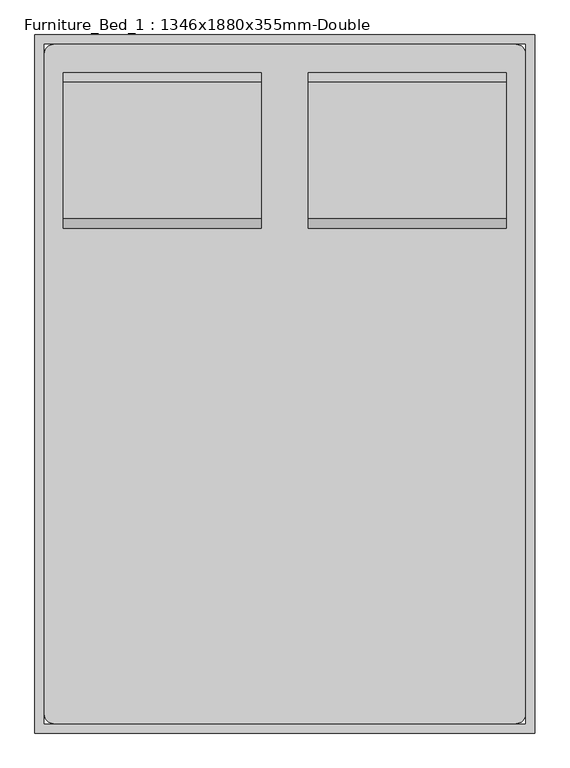
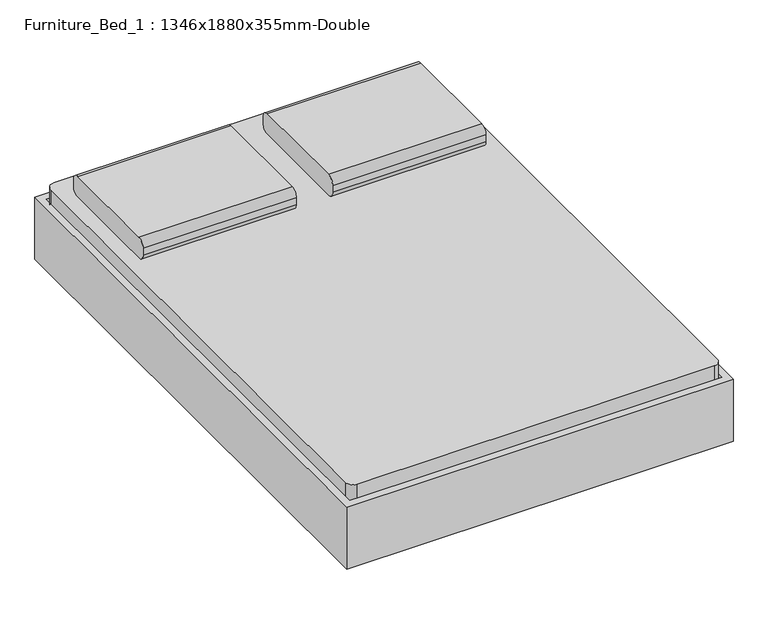
"""IFC4 building model written with IfcOpenShell, lengths in millimetres: furniture geometry, Furniture_Bed_1 : 1346x1880x355mm-Double."""

from ifc_helpers import new_model, si_unit, point, frame, frame_2d, origin, place, context, project, spatial, polyline, circle_curve, trimmed, segment, composite_curve, outline, extrude, source, transform, mapped, element, save
from ifc_brep_helpers import plane_surface, cylinder_surface, revolved_surface, advanced_brep


def furniture_bed_1_1346x1880x355mm_double_93dec6ea(model_context):
    return source(origin(), model_context, "Body", "SolidModel", [
        advanced_brep(
        [(-308.447541, -869.6295082, 196.85), (-308.447541, -869.6295082, 177.8), (-308.447541, -945.8295082, 177.8), (-308.447541, -945.8295082, 196.85), (-245.5113525, -869.6295082, 196.85), (-257.647541, -869.6295082, 177.8), (-257.647541, -945.8295082, 177.8), (-245.5113525, -945.8295082, 196.85), (-164.3115092, -869.6295082, 22.716374), (-181.5766725, -869.6295082, 14.6654962), (-181.5766725, -945.8295082, 14.6654962), (-164.3115092, -945.8295082, 22.716374), (-158.5564547, -869.6295082, 0.0), (-158.5564547, -869.6295082, 19.05), (-158.5564547, -945.8295082, 0.0), (-158.5564547, -945.8295082, 19.05), (-79.9439489, -869.6295082, 19.05), (-79.9439489, -869.6295082, 0.0), (-79.9439489, -945.8295082, 0.0), (-79.9439489, -945.8295082, 19.05), (-67.2439489, -869.6295082, 3.4029547), (-76.7689489, -869.6295082, 19.9007387), (-67.2439489, -945.8295082, 3.4029547), (-76.7689489, -945.8295082, 19.9007387), (-12.2513357, -869.6295082, 57.15), (-7.1469036, -869.6295082, 38.1), (-7.1469036, -945.8295082, 38.1), (-12.2513357, -945.8295082, 57.15), (690.5562537, -869.6295082, 57.15), (685.4518216, -869.6295082, 38.1), (685.4518216, -945.8295082, 38.1), (690.5562537, -945.8295082, 57.15), (755.0738669, -869.6295082, 19.9007387), (745.5488669, -869.6295082, 3.4029547), (745.5488669, -945.8295082, 3.4029547), (755.0738669, -945.8295082, 19.9007387), (758.2488669, -869.6295082, 0.0), (758.2488669, -869.6295082, 19.05), (758.2488669, -945.8295082, 0.0), (758.2488669, -945.8295082, 19.05), (836.8613728, -869.6295082, 19.05), (836.8613728, -869.6295082, 0.0), (836.8613728, -945.8295082, 0.0), (836.8613728, -945.8295082, 19.05), (859.8815906, -869.6295082, 14.6654962), (842.6164272, -869.6295082, 22.716374), (859.8815906, -945.8295082, 14.6654962), (842.6164272, -945.8295082, 22.716374), (923.8162705, -869.6295082, 196.85), (935.952459, -869.6295082, 177.8), (935.952459, -945.8295082, 177.8), (923.8162705, -945.8295082, 196.85), (986.752459, -869.6295082, 196.85), (986.752459, -945.8295082, 196.85), (986.752459, -945.8295082, 177.8), (986.752459, -869.6295082, 177.8)],
        [
            (0, 1),
            (1, 2),
            (2, 3),
            (3, 0),
            (0, 4),
            (4, 5),
            (5, 1),
            (5, 6),
            (6, 2),
            (6, 7),
            (7, 3),
            (7, 4),
            (4, 8),
            (8, 9),
            (9, 5),
            (9, 10),
            (10, 6),
            (10, 11),
            (11, 7),
            (11, 8),
            (12, 9, circle_curve(frame((-158.5564547, -869.6295082, 25.4), z_axis=(0.0, 1.0, 0.0), x_axis=(-0.9063077870366627, 0.0, -0.42261826174067213)), 25.4)),
            (8, 13, circle_curve(frame((-158.5564547, -869.6295082, 25.4), z_axis=(0.0, -1.0, 0.0), x_axis=(-0.9063077870366627, 0.0, -0.42261826174067213)), 6.35)),
            (13, 12),
            (14, 10, circle_curve(frame((-158.5564547, -945.8295082, 25.4), z_axis=(0.0, 1.0, 0.0), x_axis=(-0.9063077870366627, 0.0, -0.42261826174067213)), 25.4)),
            (12, 14),
            (15, 11, circle_curve(frame((-158.5564547, -945.8295082, 25.4), z_axis=(0.0, 1.0, 0.0), x_axis=(-0.9063077870366627, 0.0, -0.42261826174067213)), 6.35)),
            (14, 15),
            (15, 13),
            (13, 16),
            (16, 17),
            (17, 12),
            (17, 18),
            (18, 14),
            (18, 19),
            (19, 15),
            (19, 16),
            (20, 17, circle_curve(frame((-79.9439489, -869.6295082, 25.4), z_axis=(0.0, 1.0, 0.0), x_axis=(0.0, 0.0, -1.0)), 25.4)),
            (16, 21, circle_curve(frame((-79.9439489, -869.6295082, 25.4), z_axis=(0.0, -1.0, 0.0), x_axis=(0.0, 0.0, -1.0)), 6.35)),
            (21, 20),
            (22, 18, circle_curve(frame((-79.9439489, -945.8295082, 25.4), z_axis=(0.0, 1.0, 0.0), x_axis=(0.0, 0.0, -1.0)), 25.4)),
            (20, 22),
            (23, 19, circle_curve(frame((-79.9439489, -945.8295082, 25.4), z_axis=(0.0, 1.0, 0.0), x_axis=(0.0, 0.0, -1.0)), 6.35)),
            (22, 23),
            (23, 21),
            (21, 24),
            (24, 25),
            (25, 20),
            (25, 26),
            (26, 22),
            (26, 27),
            (27, 23),
            (27, 24),
            (24, 28),
            (28, 29),
            (29, 25),
            (29, 30),
            (30, 26),
            (30, 31),
            (31, 27),
            (31, 28),
            (28, 32),
            (32, 33),
            (33, 29),
            (33, 34),
            (34, 30),
            (34, 35),
            (35, 31),
            (35, 32),
            (36, 33, circle_curve(frame((758.2488669, -869.6295082, 25.4), z_axis=(0.0, 1.0, 0.0), x_axis=(-0.5000000000000486, 0.0, -0.8660254037844105)), 25.4)),
            (32, 37, circle_curve(frame((758.2488669, -869.6295082, 25.4), z_axis=(0.0, -1.0, 0.0), x_axis=(-0.5000000000000486, 0.0, -0.8660254037844105)), 6.35)),
            (37, 36),
            (38, 34, circle_curve(frame((758.2488669, -945.8295082, 25.4), z_axis=(0.0, 1.0, 0.0), x_axis=(-0.5000000000000486, 0.0, -0.8660254037844105)), 25.4)),
            (36, 38),
            (39, 35, circle_curve(frame((758.2488669, -945.8295082, 25.4), z_axis=(0.0, 1.0, 0.0), x_axis=(-0.5000000000000486, 0.0, -0.8660254037844105)), 6.35)),
            (38, 39),
            (39, 37),
            (37, 40),
            (40, 41),
            (41, 36),
            (41, 42),
            (42, 38),
            (42, 43),
            (43, 39),
            (43, 40),
            (44, 41, circle_curve(frame((836.8613728, -869.6295082, 25.4), z_axis=(0.0, 1.0, 0.0), x_axis=(0.0, 0.0, -1.0)), 25.4)),
            (40, 45, circle_curve(frame((836.8613728, -869.6295082, 25.4), z_axis=(0.0, -1.0, 0.0), x_axis=(0.0, 0.0, -1.0)), 6.35)),
            (45, 44),
            (46, 42, circle_curve(frame((836.8613728, -945.8295082, 25.4), z_axis=(0.0, 1.0, 0.0), x_axis=(0.0, 0.0, -1.0)), 25.4)),
            (44, 46),
            (47, 43, circle_curve(frame((836.8613728, -945.8295082, 25.4), z_axis=(0.0, 1.0, 0.0), x_axis=(0.0, 0.0, -1.0)), 6.35)),
            (46, 47),
            (47, 45),
            (45, 48),
            (48, 49),
            (49, 44),
            (49, 50),
            (50, 46),
            (50, 51),
            (51, 47),
            (51, 48),
            (52, 53),
            (53, 54),
            (54, 55),
            (55, 52),
            (48, 52),
            (55, 49),
            (54, 50),
            (53, 51),
        ],
        [
            plane_surface(frame((-308.447541, -1174.4295082, -127.5947323), z_axis=(-1.0, 0.0, 0.0), x_axis=(0.0, 1.0, 0.0))),
            plane_surface(frame((-308.447541, -869.6295082, 196.85), z_axis=(0.0, 1.0, 0.0), x_axis=(1.0, 0.0, 0.0))),
            plane_surface(frame((-308.447541, -869.6295082, 177.8), z_axis=(0.0, 0.0, -1.0), x_axis=(1.0, 0.0, 0.0))),
            plane_surface(frame((-308.447541, -945.8295082, 177.8), z_axis=(0.0, -1.0, 0.0), x_axis=(1.0, 0.0, 0.0))),
            plane_surface(frame((-308.447541, -945.8295082, 196.85), z_axis=(0.0, 0.0, 1.0), x_axis=(1.0, 0.0, 0.0))),
            plane_surface(frame((-245.5113525, -869.6295082, 196.85), z_axis=(0.0, 1.0, 0.0), x_axis=(0.42261826174067146, 0.0, -0.906307787036663))),
            plane_surface(frame((-257.647541, -869.6295082, 177.8), z_axis=(-0.9063077870366631, 0.0, -0.4226182617406713), x_axis=(0.4226182617406713, 0.0, -0.9063077870366631))),
            plane_surface(frame((-257.647541, -945.8295082, 177.8), z_axis=(0.0, -1.0, 0.0), x_axis=(0.4226182617406716, 0.0, -0.9063077870366629))),
            plane_surface(frame((-245.5113525, -945.8295082, 196.85), z_axis=(0.906307787036663, 0.0, 0.4226182617406716), x_axis=(0.4226182617406716, 0.0, -0.906307787036663))),
            plane_surface(frame((-158.5564547, -869.6295082, 25.4), z_axis=(0.0, 1.0, 0.0), x_axis=(-0.9063077870366627, 0.0, -0.42261826174067213))),
            cylinder_surface(frame((-158.5564547, -1174.4295082, 25.4), z_axis=(0.0, -1.0, 0.0), x_axis=(-0.9063077870366627, 0.0, -0.42261826174067213)), 25.4),
            plane_surface(frame((-158.5564547, -945.8295082, 25.4), z_axis=(0.0, -1.0, 0.0), x_axis=(-0.9063077870366627, 0.0, -0.42261826174067213))),
            revolved_surface(polyline([(-164.31150914768278, -945.8295082, 22.716374037946732), (-164.31150914768278, -869.6295082, 22.716374037946732)]), (-158.5564547, -1174.4295082, 25.4), (0.0, -1.0, 0.0)),
            plane_surface(frame((-158.5564547, -869.6295082, 19.05), z_axis=(0.0, 1.0, 0.0), x_axis=(1.0, 0.0, 0.0))),
            plane_surface(frame((-158.5564547, -869.6295082, 0.0), z_axis=(0.0, 0.0, -1.0), x_axis=(1.0, 0.0, 0.0))),
            plane_surface(frame((-158.5564547, -945.8295082, 0.0), z_axis=(0.0, -1.0, 0.0), x_axis=(1.0, 0.0, 0.0))),
            plane_surface(frame((-158.5564547, -945.8295082, 19.05), z_axis=(0.0, 0.0, 1.0), x_axis=(1.0, 0.0, 0.0))),
            plane_surface(frame((-79.9439489, -869.6295082, 25.4), z_axis=(0.0, 1.0, 0.0), x_axis=(0.0, 0.0, -1.0))),
            cylinder_surface(frame((-79.9439489, -1174.4295082, 25.4), z_axis=(0.0, -1.0, 0.0), x_axis=(0.0, 0.0, -1.0)), 25.4),
            plane_surface(frame((-79.9439489, -945.8295082, 25.4), z_axis=(0.0, -1.0, 0.0), x_axis=(0.0, 0.0, -1.0))),
            revolved_surface(polyline([(-79.9439489, -945.8295082, 19.049999999999997), (-79.9439489, -869.6295082, 19.049999999999997)]), (-79.9439489, -1174.4295082, 25.4), (0.0, -1.0, 0.0)),
            plane_surface(frame((-76.7689489, -869.6295082, 19.9007387), z_axis=(0.0, 1.0, 0.0), x_axis=(0.8660254037844782, 0.0, 0.4999999999999314))),
            plane_surface(frame((-67.2439489, -869.6295082, 3.4029547), z_axis=(0.49999999999993133, 0.0, -0.8660254037844783), x_axis=(0.8660254037844783, 0.0, 0.49999999999993133))),
            plane_surface(frame((-67.2439489, -945.8295082, 3.4029547), z_axis=(0.0, -1.0, 0.0), x_axis=(0.8660254037844785, 0.0, 0.499999999999931))),
            plane_surface(frame((-76.7689489, -945.8295082, 19.9007387), z_axis=(-0.49999999999993144, 0.0, 0.8660254037844782), x_axis=(0.8660254037844782, 0.0, 0.49999999999993144))),
            plane_surface(frame((-12.2513357, -869.6295082, 57.15), z_axis=(0.0, 1.0, 0.0), x_axis=(1.0, 0.0, 0.0))),
            plane_surface(frame((-7.1469036, -869.6295082, 38.1), z_axis=(0.0, 0.0, -1.0), x_axis=(1.0, 0.0, 0.0))),
            plane_surface(frame((-7.1469036, -945.8295082, 38.1), z_axis=(0.0, -1.0, 0.0), x_axis=(1.0, 0.0, 0.0))),
            plane_surface(frame((-12.2513357, -945.8295082, 57.15), z_axis=(0.0, 0.0, 1.0), x_axis=(1.0, 0.0, 0.0))),
            plane_surface(frame((690.5562537, -869.6295082, 57.15), z_axis=(0.0, 1.0, 0.0), x_axis=(0.8660254037844104, 0.0, -0.5000000000000491))),
            plane_surface(frame((685.4518216, -869.6295082, 38.1), z_axis=(-0.5000000000000484, 0.0, -0.8660254037844108), x_axis=(0.8660254037844108, 0.0, -0.5000000000000484))),
            plane_surface(frame((685.4518216, -945.8295082, 38.1), z_axis=(0.0, -1.0000000000000002, 0.0), x_axis=(0.8660254037844103, 0.0, -0.5000000000000493))),
            plane_surface(frame((690.5562537, -945.8295082, 57.15), z_axis=(0.5000000000000485, 0.0, 0.8660254037844106), x_axis=(0.8660254037844106, 0.0, -0.5000000000000485))),
            plane_surface(frame((758.2488669, -869.6295082, 25.4), z_axis=(0.0, 1.0000000000000002, 0.0), x_axis=(-0.5000000000000487, 0.0, -0.8660254037844106))),
            cylinder_surface(frame((758.2488669, -1174.4295082, 25.4), z_axis=(0.0, -1.0, 0.0), x_axis=(-0.5000000000000486, 0.0, -0.8660254037844105)), 25.4),
            plane_surface(frame((758.2488669, -945.8295082, 25.4), z_axis=(0.0, -1.0000000000000002, 0.0), x_axis=(-0.5000000000000487, 0.0, -0.8660254037844106))),
            revolved_surface(polyline([(755.0738668999998, -945.8295082, 19.900738685968992), (755.0738668999998, -869.6295082, 19.900738685968992)]), (758.2488669, -1174.4295082, 25.4), (0.0, -1.0, 0.0)),
            plane_surface(frame((758.2488669, -869.6295082, 19.05), z_axis=(0.0, 1.0, 0.0), x_axis=(1.0, 0.0, 0.0))),
            plane_surface(frame((758.2488669, -869.6295082, 0.0), z_axis=(0.0, 0.0, -1.0), x_axis=(1.0, 0.0, 0.0))),
            plane_surface(frame((758.2488669, -945.8295082, 0.0), z_axis=(0.0, -1.0, 0.0), x_axis=(1.0, 0.0, 0.0))),
            plane_surface(frame((758.2488669, -945.8295082, 19.05), z_axis=(0.0, 0.0, 1.0), x_axis=(1.0, 0.0, 0.0))),
            plane_surface(frame((836.8613728, -869.6295082, 25.4), z_axis=(0.0, 1.0, 0.0), x_axis=(0.0, 0.0, -1.0))),
            cylinder_surface(frame((836.8613728, -1174.4295082, 25.4), z_axis=(0.0, -1.0, 0.0), x_axis=(0.0, 0.0, -1.0)), 25.4),
            plane_surface(frame((836.8613728, -945.8295082, 25.4), z_axis=(0.0, -1.0, 0.0), x_axis=(0.0, 0.0, -1.0))),
            revolved_surface(polyline([(836.8613728, -945.8295082, 19.049999999999997), (836.8613728, -869.6295082, 19.049999999999997)]), (836.8613728, -1174.4295082, 25.4), (0.0, -1.0, 0.0)),
            plane_surface(frame((842.6164272, -869.6295082, 22.716374), z_axis=(0.0, 1.0, 0.0), x_axis=(0.4226182617405402, 0.0, 0.9063077870367242))),
            plane_surface(frame((859.8815906, -869.6295082, 14.6654962), z_axis=(0.9063077870367245, 0.0, -0.42261826174053974), x_axis=(0.42261826174053974, 0.0, 0.9063077870367245))),
            plane_surface(frame((859.8815906, -945.8295082, 14.6654962), z_axis=(0.0, -1.0000000000000002, 0.0), x_axis=(0.42261826174053974, 0.0, 0.9063077870367245))),
            plane_surface(frame((842.6164272, -945.8295082, 22.716374), z_axis=(-0.9063077870367247, 0.0, 0.4226182617405394), x_axis=(0.4226182617405394, 0.0, 0.9063077870367247))),
            plane_surface(frame((986.752459, -1174.4295082, -127.5947323), z_axis=(1.0, 0.0, 0.0), x_axis=(0.0, 1.0, 0.0))),
            plane_surface(frame((923.8162705, -869.6295082, 196.85), z_axis=(0.0, 1.0, 0.0), x_axis=(1.0, 0.0, 0.0))),
            plane_surface(frame((935.952459, -869.6295082, 177.8), z_axis=(0.0, 0.0, -1.0), x_axis=(1.0, 0.0, 0.0))),
            plane_surface(frame((935.952459, -945.8295082, 177.8), z_axis=(0.0, -1.0, 0.0), x_axis=(1.0, 0.0, 0.0))),
            plane_surface(frame((923.8162705, -945.8295082, 196.85), z_axis=(0.0, 0.0, 1.0), x_axis=(1.0, 0.0, 0.0))),
        ],
        [
            (0, [[1, 2, 3, 4]]),
            (1, [[-1, 5, 6, 7]]),
            (2, [[-2, -7, 8, 9]]),
            (3, [[-3, -9, 10, 11]]),
            (4, [[-4, -11, 12, -5]]),
            (5, [[-6, 13, 14, 15]]),
            (6, [[-8, -15, 16, 17]]),
            (7, [[-10, -17, 18, 19]]),
            (8, [[-12, -19, 20, -13]]),
            (9, [[21, -14, 22, 23]]),
            (10, [[24, -16, -21, 25]]),
            (11, [[26, -18, -24, 27]]),
            (12, [[-22, -20, -26, 28]]),
            (13, [[-23, 29, 30, 31]]),
            (14, [[-25, -31, 32, 33]]),
            (15, [[-27, -33, 34, 35]]),
            (16, [[-28, -35, 36, -29]]),
            (17, [[37, -30, 38, 39]]),
            (18, [[40, -32, -37, 41]]),
            (19, [[42, -34, -40, 43]]),
            (20, [[-38, -36, -42, 44]]),
            (21, [[-39, 45, 46, 47]]),
            (22, [[-41, -47, 48, 49]]),
            (23, [[-43, -49, 50, 51]]),
            (24, [[-44, -51, 52, -45]]),
            (25, [[-46, 53, 54, 55]]),
            (26, [[-48, -55, 56, 57]]),
            (27, [[-50, -57, 58, 59]]),
            (28, [[-52, -59, 60, -53]]),
            (29, [[-54, 61, 62, 63]]),
            (30, [[-56, -63, 64, 65]]),
            (31, [[-58, -65, 66, 67]]),
            (32, [[-60, -67, 68, -61]]),
            (33, [[69, -62, 70, 71]]),
            (34, [[72, -64, -69, 73]]),
            (35, [[74, -66, -72, 75]]),
            (36, [[-70, -68, -74, 76]]),
            (37, [[-71, 77, 78, 79]]),
            (38, [[-73, -79, 80, 81]]),
            (39, [[-75, -81, 82, 83]]),
            (40, [[-76, -83, 84, -77]]),
            (41, [[85, -78, 86, 87]]),
            (42, [[88, -80, -85, 89]]),
            (43, [[90, -82, -88, 91]]),
            (44, [[-86, -84, -90, 92]]),
            (45, [[-87, 93, 94, 95]]),
            (46, [[-89, -95, 96, 97]]),
            (47, [[-91, -97, 98, 99]]),
            (48, [[-92, -99, 100, -93]]),
            (49, [[101, 102, 103, 104]]),
            (50, [[-94, 105, -104, 106]]),
            (51, [[-96, -106, -103, 107]]),
            (52, [[-98, -107, -102, 108]]),
            (53, [[-100, -108, -101, -105]]),
        ],
    ),
        extrude(outline(composite_curve([segment(polyline([(-283.047541, 680.1704918), (961.352459, 680.1704918)]), True, "CONTINUOUS"), segment(trimmed(circle_curve(frame_2d((961.352459, 654.7704918)), 25.4), [point((961.352459, 680.1704918))], [point((986.752459, 654.7704918))], False, "CARTESIAN"), True, "CONTINUOUS"), segment(polyline([(986.752459, 654.7704918), (986.752459, -1123.6295082)]), True, "CONTINUOUS"), segment(trimmed(circle_curve(frame_2d((961.352459, -1123.6295082)), 25.4), [point((986.752459, -1123.6295082))], [point((961.352459, -1149.0295082))], False, "CARTESIAN"), True, "CONTINUOUS"), segment(polyline([(961.352459, -1149.0295082), (-283.047541, -1149.0295082)]), True, "CONTINUOUS"), segment(trimmed(circle_curve(frame_2d((-283.047541, -1123.6295082)), 25.4), [point((-283.047541, -1149.0295082))], [point((-308.447541, -1123.6295082))], False, "CARTESIAN"), True, "CONTINUOUS"), segment(polyline([(-308.447541, -1123.6295082), (-308.447541, 654.7704918)]), True, "CONTINUOUS"), segment(trimmed(circle_curve(frame_2d((-283.047541, 654.7704918)), 25.4), [point((-308.447541, 654.7704918))], [point((-283.047541, 680.1704918))], False, "CARTESIAN"), True, "CONTINUOUS")], self_intersect=False)), frame((0.0, 0.0, 203.2), z_axis=(0.0, 0.0, 1.0), x_axis=(1.0, 0.0, 0.0)), (0.0, 0.0, 1.0), 203.2),
        advanced_brep(
        [(-308.1231784, 451.5704918, 177.8), (-308.1231784, 375.3704918, 177.8), (-308.1231784, 375.3704918, 196.85), (-308.1231784, 451.5704918, 196.85), (-257.3231784, 451.5704918, 177.8), (-257.3231784, 375.3704918, 177.8), (-245.1869899, 375.3704918, 196.85), (-245.1869899, 451.5704918, 196.85), (-181.2523099, 451.5704918, 14.6654962), (-181.2523099, 375.3704918, 14.6654962), (-163.9871466, 375.3704918, 22.716374), (-163.9871466, 451.5704918, 22.716374), (-158.2320921, 375.3704918, 0.0), (-158.2320921, 451.5704918, 0.0), (-158.2320921, 375.3704918, 19.05), (-158.2320921, 451.5704918, 19.05), (-79.6195862, 451.5704918, 0.0), (-79.6195862, 375.3704918, 0.0), (-79.6195862, 375.3704918, 19.05), (-79.6195862, 451.5704918, 19.05), (-66.9195862, 375.3704918, 3.4029547), (-66.9195862, 451.5704918, 3.4029547), (-76.4445862, 375.3704918, 19.9007387), (-76.4445862, 451.5704918, 19.9007387), (-6.822541, 451.5704918, 38.1), (-6.822541, 375.3704918, 38.1), (-11.9269731, 375.3704918, 57.15), (-11.9269731, 451.5704918, 57.15), (685.4518216, 451.5704918, 38.1), (685.4518216, 375.3704918, 38.1), (690.5562537, 375.3704918, 57.15), (690.5562537, 451.5704918, 57.15), (745.5488669, 451.5704918, 3.4029547), (745.5488669, 375.3704918, 3.4029547), (755.0738669, 375.3704918, 19.9007387), (755.0738669, 451.5704918, 19.9007387), (758.2488669, 375.3704918, 0.0), (758.2488669, 451.5704918, 0.0), (758.2488669, 375.3704918, 19.05), (758.2488669, 451.5704918, 19.05), (836.8613728, 451.5704918, 0.0), (836.8613728, 375.3704918, 0.0), (836.8613728, 375.3704918, 19.05), (836.8613728, 451.5704918, 19.05), (859.8815906, 375.3704918, 14.6654962), (859.8815906, 451.5704918, 14.6654962), (842.6164272, 375.3704918, 22.716374), (842.6164272, 451.5704918, 22.716374), (935.952459, 451.5704918, 177.8), (935.952459, 375.3704918, 177.8), (923.8162705, 375.3704918, 196.85), (923.8162705, 451.5704918, 196.85), (986.752459, 451.5704918, 177.8), (986.752459, 451.5704918, 196.85), (986.752459, 375.3704918, 196.85), (986.752459, 375.3704918, 177.8)],
        [
            (0, 1),
            (1, 2),
            (2, 3),
            (3, 0),
            (0, 4),
            (4, 5),
            (5, 1),
            (5, 6),
            (6, 2),
            (6, 7),
            (7, 3),
            (7, 4),
            (4, 8),
            (8, 9),
            (9, 5),
            (9, 10),
            (10, 6),
            (10, 11),
            (11, 7),
            (11, 8),
            (12, 9, circle_curve(frame((-158.2320921, 375.3704918, 25.4), z_axis=(0.0, 1.0, 0.0), x_axis=(-0.906307787036649, 0.0, -0.4226182617407015)), 25.4)),
            (8, 13, circle_curve(frame((-158.2320921, 451.5704918, 25.4), z_axis=(0.0, -1.0, 0.0), x_axis=(-0.906307787036649, 0.0, -0.4226182617407015)), 25.4)),
            (13, 12),
            (14, 10, circle_curve(frame((-158.2320921, 375.3704918, 25.4), z_axis=(0.0, 1.0, 0.0), x_axis=(-0.906307787036649, 0.0, -0.4226182617407015)), 6.35)),
            (12, 14),
            (15, 11, circle_curve(frame((-158.2320921, 451.5704918, 25.4), z_axis=(0.0, 1.0, 0.0), x_axis=(-0.906307787036649, 0.0, -0.4226182617407015)), 6.35)),
            (14, 15),
            (15, 13),
            (13, 16),
            (16, 17),
            (17, 12),
            (17, 18),
            (18, 14),
            (18, 19),
            (19, 15),
            (19, 16),
            (20, 17, circle_curve(frame((-79.6195862, 375.3704918, 25.4), z_axis=(0.0, 1.0, 0.0), x_axis=(0.0, 0.0, -1.0)), 25.4)),
            (16, 21, circle_curve(frame((-79.6195862, 451.5704918, 25.4), z_axis=(0.0, -1.0, 0.0), x_axis=(0.0, 0.0, -1.0)), 25.4)),
            (21, 20),
            (22, 18, circle_curve(frame((-79.6195862, 375.3704918, 25.4), z_axis=(0.0, 1.0, 0.0), x_axis=(0.0, 0.0, -1.0)), 6.35)),
            (20, 22),
            (23, 19, circle_curve(frame((-79.6195862, 451.5704918, 25.4), z_axis=(0.0, 1.0, 0.0), x_axis=(0.0, 0.0, -1.0)), 6.35)),
            (22, 23),
            (23, 21),
            (21, 24),
            (24, 25),
            (25, 20),
            (25, 26),
            (26, 22),
            (26, 27),
            (27, 23),
            (27, 24),
            (24, 28),
            (28, 29),
            (29, 25),
            (29, 30),
            (30, 26),
            (30, 31),
            (31, 27),
            (31, 28),
            (28, 32),
            (32, 33),
            (33, 29),
            (33, 34),
            (34, 30),
            (34, 35),
            (35, 31),
            (35, 32),
            (36, 33, circle_curve(frame((758.2488669, 375.3704918, 25.4), z_axis=(0.0, 1.0, 0.0), x_axis=(-0.5000000000000444, 0.0, -0.866025403784413)), 25.4)),
            (32, 37, circle_curve(frame((758.2488669, 451.5704918, 25.4), z_axis=(0.0, -1.0, 0.0), x_axis=(-0.5000000000000444, 0.0, -0.866025403784413)), 25.4)),
            (37, 36),
            (38, 34, circle_curve(frame((758.2488669, 375.3704918, 25.4), z_axis=(0.0, 1.0, 0.0), x_axis=(-0.5000000000000444, 0.0, -0.866025403784413)), 6.35)),
            (36, 38),
            (39, 35, circle_curve(frame((758.2488669, 451.5704918, 25.4), z_axis=(0.0, 1.0, 0.0), x_axis=(-0.5000000000000444, 0.0, -0.866025403784413)), 6.35)),
            (38, 39),
            (39, 37),
            (37, 40),
            (40, 41),
            (41, 36),
            (41, 42),
            (42, 38),
            (42, 43),
            (43, 39),
            (43, 40),
            (44, 41, circle_curve(frame((836.8613728, 375.3704918, 25.4), z_axis=(0.0, 1.0, 0.0), x_axis=(0.0, 0.0, -1.0)), 25.4)),
            (40, 45, circle_curve(frame((836.8613728, 451.5704918, 25.4), z_axis=(0.0, -1.0, 0.0), x_axis=(0.0, 0.0, -1.0)), 25.4)),
            (45, 44),
            (46, 42, circle_curve(frame((836.8613728, 375.3704918, 25.4), z_axis=(0.0, 1.0, 0.0), x_axis=(0.0, 0.0, -1.0)), 6.35)),
            (44, 46),
            (47, 43, circle_curve(frame((836.8613728, 451.5704918, 25.4), z_axis=(0.0, 1.0, 0.0), x_axis=(0.0, 0.0, -1.0)), 6.35)),
            (46, 47),
            (47, 45),
            (45, 48),
            (48, 49),
            (49, 44),
            (49, 50),
            (50, 46),
            (50, 51),
            (51, 47),
            (51, 48),
            (52, 53),
            (53, 54),
            (54, 55),
            (55, 52),
            (48, 52),
            (55, 49),
            (54, 50),
            (53, 51),
        ],
        [
            plane_surface(frame((-308.1231784, 705.5704918, -152.9490627), z_axis=(-1.0, 0.0, 0.0), x_axis=(0.0, 1.0, 0.0))),
            plane_surface(frame((-308.1231784, 451.5704918, 177.8), z_axis=(0.0, 0.0, -1.0), x_axis=(1.0, 0.0, 0.0))),
            plane_surface(frame((-308.1231784, 375.3704918, 177.8), z_axis=(0.0, -1.0, 0.0), x_axis=(1.0, 0.0, 0.0))),
            plane_surface(frame((-308.1231784, 375.3704918, 196.85), z_axis=(0.0, 0.0, 1.0), x_axis=(1.0, 0.0, 0.0))),
            plane_surface(frame((-308.1231784, 451.5704918, 196.85), z_axis=(0.0, 1.0, 0.0), x_axis=(1.0, 0.0, 0.0))),
            plane_surface(frame((-257.3231784, 451.5704918, 177.8), z_axis=(-0.9063077870366483, 0.0, -0.4226182617407031), x_axis=(0.4226182617407031, 0.0, -0.9063077870366483))),
            plane_surface(frame((-257.3231784, 375.3704918, 177.8), z_axis=(0.0, -1.0, 0.0), x_axis=(0.4226182617407027, 0.0, -0.9063077870366485))),
            plane_surface(frame((-245.1869899, 375.3704918, 196.85), z_axis=(0.9063077870366484, 0.0, 0.4226182617407029), x_axis=(0.4226182617407029, 0.0, -0.9063077870366484))),
            plane_surface(frame((-245.1869899, 451.5704918, 196.85), z_axis=(0.0, 1.0, 0.0), x_axis=(0.4226182617407027, 0.0, -0.9063077870366485))),
            cylinder_surface(frame((-158.2320921, 705.5704918, 25.4), z_axis=(0.0, -1.0, 0.0), x_axis=(-0.906307787036649, 0.0, -0.4226182617407015)), 25.4),
            plane_surface(frame((-158.2320921, 375.3704918, 25.4), z_axis=(0.0, -1.0, 0.0), x_axis=(-0.906307787036649, 0.0, -0.4226182617407015))),
            revolved_surface(polyline([(-163.9871465476827, 375.3704918, 22.716374037946544), (-163.9871465476827, 451.5704918, 22.716374037946544)]), (-158.2320921, 705.5704918, 25.4), (0.0, -1.0, 0.0)),
            plane_surface(frame((-158.2320921, 451.5704918, 25.4), z_axis=(0.0, 1.0, 0.0), x_axis=(-0.906307787036649, 0.0, -0.4226182617407015))),
            plane_surface(frame((-158.2320921, 451.5704918, 0.0), z_axis=(0.0, 0.0, -1.0), x_axis=(1.0, 0.0, 0.0))),
            plane_surface(frame((-158.2320921, 375.3704918, 0.0), z_axis=(0.0, -1.0, 0.0), x_axis=(1.0, 0.0, 0.0))),
            plane_surface(frame((-158.2320921, 375.3704918, 19.05), z_axis=(0.0, 0.0, 1.0), x_axis=(1.0, 0.0, 0.0))),
            plane_surface(frame((-158.2320921, 451.5704918, 19.05), z_axis=(0.0, 1.0, 0.0), x_axis=(1.0, 0.0, 0.0))),
            cylinder_surface(frame((-79.6195862, 705.5704918, 25.4), z_axis=(0.0, -1.0, 0.0), x_axis=(0.0, 0.0, -1.0)), 25.4),
            plane_surface(frame((-79.6195862, 375.3704918, 25.4), z_axis=(0.0, -1.0, 0.0), x_axis=(0.0, 0.0, -1.0))),
            revolved_surface(polyline([(-79.6195862, 375.3704918, 19.049999999999997), (-79.6195862, 451.5704918, 19.049999999999997)]), (-79.6195862, 705.5704918, 25.4), (0.0, -1.0, 0.0)),
            plane_surface(frame((-79.6195862, 451.5704918, 25.4), z_axis=(0.0, 1.0, 0.0), x_axis=(0.0, 0.0, -1.0))),
            plane_surface(frame((-66.9195862, 451.5704918, 3.4029547), z_axis=(0.4999999999998771, 0.0, -0.8660254037845097), x_axis=(0.8660254037845097, 0.0, 0.4999999999998771))),
            plane_surface(frame((-66.9195862, 375.3704918, 3.4029547), z_axis=(0.0, -1.0000000000000002, 0.0), x_axis=(0.8660254037845102, 0.0, 0.49999999999987627))),
            plane_surface(frame((-76.4445862, 375.3704918, 19.9007387), z_axis=(-0.49999999999987643, 0.0, 0.86602540378451), x_axis=(0.86602540378451, 0.0, 0.49999999999987643))),
            plane_surface(frame((-76.4445862, 451.5704918, 19.9007387), z_axis=(0.0, 1.0, 0.0), x_axis=(0.8660254037845102, 0.0, 0.4999999999998761))),
            plane_surface(frame((-6.822541, 451.5704918, 38.1), z_axis=(0.0, 0.0, -1.0), x_axis=(1.0, 0.0, 0.0))),
            plane_surface(frame((-6.822541, 375.3704918, 38.1), z_axis=(0.0, -1.0, 0.0), x_axis=(1.0, 0.0, 0.0))),
            plane_surface(frame((-11.9269731, 375.3704918, 57.15), z_axis=(0.0, 0.0, 1.0), x_axis=(1.0, 0.0, 0.0))),
            plane_surface(frame((-11.9269731, 451.5704918, 57.15), z_axis=(0.0, 1.0, 0.0), x_axis=(1.0, 0.0, 0.0))),
            plane_surface(frame((685.4518216, 451.5704918, 38.1), z_axis=(-0.5000000000000445, 0.0, -0.866025403784413), x_axis=(0.866025403784413, 0.0, -0.5000000000000445))),
            plane_surface(frame((685.4518216, 375.3704918, 38.1), z_axis=(0.0, -1.0, 0.0), x_axis=(0.8660254037844118, 0.0, -0.5000000000000464))),
            plane_surface(frame((690.5562537, 375.3704918, 57.15), z_axis=(0.5000000000000461, 0.0, 0.8660254037844121), x_axis=(0.8660254037844121, 0.0, -0.5000000000000461))),
            plane_surface(frame((690.5562537, 451.5704918, 57.15), z_axis=(0.0, 1.0, 0.0), x_axis=(0.8660254037844126, 0.0, -0.5000000000000452))),
            cylinder_surface(frame((758.2488669, 705.5704918, 25.4), z_axis=(0.0, -1.0, 0.0), x_axis=(-0.5000000000000444, 0.0, -0.866025403784413)), 25.4),
            plane_surface(frame((758.2488669, 375.3704918, 25.4), z_axis=(0.0, -1.0000000000000002, 0.0), x_axis=(-0.5000000000000445, 0.0, -0.8660254037844131))),
            revolved_surface(polyline([(755.0738668999998, 375.3704918, 19.900738685968975), (755.0738668999998, 451.5704918, 19.900738685968975)]), (758.2488669, 705.5704918, 25.4), (0.0, -1.0, 0.0)),
            plane_surface(frame((758.2488669, 451.5704918, 25.4), z_axis=(0.0, 1.0000000000000002, 0.0), x_axis=(-0.5000000000000445, 0.0, -0.8660254037844131))),
            plane_surface(frame((758.2488669, 451.5704918, 0.0), z_axis=(0.0, 0.0, -1.0), x_axis=(1.0, 0.0, 0.0))),
            plane_surface(frame((758.2488669, 375.3704918, 0.0), z_axis=(0.0, -1.0, 0.0), x_axis=(1.0, 0.0, 0.0))),
            plane_surface(frame((758.2488669, 375.3704918, 19.05), z_axis=(0.0, 0.0, 1.0), x_axis=(1.0, 0.0, 0.0))),
            plane_surface(frame((758.2488669, 451.5704918, 19.05), z_axis=(0.0, 1.0, 0.0), x_axis=(1.0, 0.0, 0.0))),
            cylinder_surface(frame((836.8613728, 705.5704918, 25.4), z_axis=(0.0, -1.0, 0.0), x_axis=(0.0, 0.0, -1.0)), 25.4),
            plane_surface(frame((836.8613728, 375.3704918, 25.4), z_axis=(0.0, -1.0, 0.0), x_axis=(0.0, 0.0, -1.0))),
            revolved_surface(polyline([(836.8613728, 375.3704918, 19.049999999999997), (836.8613728, 451.5704918, 19.049999999999997)]), (836.8613728, 705.5704918, 25.4), (0.0, -1.0, 0.0)),
            plane_surface(frame((836.8613728, 451.5704918, 25.4), z_axis=(0.0, 1.0, 0.0), x_axis=(0.0, 0.0, -1.0))),
            plane_surface(frame((859.8815906, 451.5704918, 14.6654962), z_axis=(0.9063077870366807, 0.0, -0.42261826174063377), x_axis=(0.42261826174063377, 0.0, 0.9063077870366807))),
            plane_surface(frame((859.8815906, 375.3704918, 14.6654962), z_axis=(0.0, -1.0, 0.0), x_axis=(0.422618261740633, 0.0, 0.9063077870366809))),
            plane_surface(frame((842.6164272, 375.3704918, 22.716374), z_axis=(-0.9063077870366809, 0.0, 0.4226182617406331), x_axis=(0.4226182617406331, 0.0, 0.9063077870366809))),
            plane_surface(frame((842.6164272, 451.5704918, 22.716374), z_axis=(0.0, 1.0, 0.0), x_axis=(0.42261826174063294, 0.0, 0.906307787036681))),
            plane_surface(frame((986.752459, 705.5704918, -152.9490627), z_axis=(1.0, 0.0, 0.0), x_axis=(0.0, 1.0, 0.0))),
            plane_surface(frame((935.952459, 451.5704918, 177.8), z_axis=(0.0, 0.0, -1.0), x_axis=(1.0, 0.0, 0.0))),
            plane_surface(frame((935.952459, 375.3704918, 177.8), z_axis=(0.0, -1.0, 0.0), x_axis=(1.0, 0.0, 0.0))),
            plane_surface(frame((923.8162705, 375.3704918, 196.85), z_axis=(0.0, 0.0, 1.0), x_axis=(1.0, 0.0, 0.0))),
            plane_surface(frame((923.8162705, 451.5704918, 196.85), z_axis=(0.0, 1.0, 0.0), x_axis=(1.0, 0.0, 0.0))),
        ],
        [
            (0, [[1, 2, 3, 4]]),
            (1, [[-1, 5, 6, 7]]),
            (2, [[-2, -7, 8, 9]]),
            (3, [[-3, -9, 10, 11]]),
            (4, [[-4, -11, 12, -5]]),
            (5, [[-6, 13, 14, 15]]),
            (6, [[-8, -15, 16, 17]]),
            (7, [[-10, -17, 18, 19]]),
            (8, [[-12, -19, 20, -13]]),
            (9, [[21, -14, 22, 23]]),
            (10, [[24, -16, -21, 25]]),
            (11, [[26, -18, -24, 27]]),
            (12, [[-22, -20, -26, 28]]),
            (13, [[-23, 29, 30, 31]]),
            (14, [[-25, -31, 32, 33]]),
            (15, [[-27, -33, 34, 35]]),
            (16, [[-28, -35, 36, -29]]),
            (17, [[37, -30, 38, 39]]),
            (18, [[40, -32, -37, 41]]),
            (19, [[42, -34, -40, 43]]),
            (20, [[-38, -36, -42, 44]]),
            (21, [[-39, 45, 46, 47]]),
            (22, [[-41, -47, 48, 49]]),
            (23, [[-43, -49, 50, 51]]),
            (24, [[-44, -51, 52, -45]]),
            (25, [[-46, 53, 54, 55]]),
            (26, [[-48, -55, 56, 57]]),
            (27, [[-50, -57, 58, 59]]),
            (28, [[-52, -59, 60, -53]]),
            (29, [[-54, 61, 62, 63]]),
            (30, [[-56, -63, 64, 65]]),
            (31, [[-58, -65, 66, 67]]),
            (32, [[-60, -67, 68, -61]]),
            (33, [[69, -62, 70, 71]]),
            (34, [[72, -64, -69, 73]]),
            (35, [[74, -66, -72, 75]]),
            (36, [[-70, -68, -74, 76]]),
            (37, [[-71, 77, 78, 79]]),
            (38, [[-73, -79, 80, 81]]),
            (39, [[-75, -81, 82, 83]]),
            (40, [[-76, -83, 84, -77]]),
            (41, [[85, -78, 86, 87]]),
            (42, [[88, -80, -85, 89]]),
            (43, [[90, -82, -88, 91]]),
            (44, [[-86, -84, -90, 92]]),
            (45, [[-87, 93, 94, 95]]),
            (46, [[-89, -95, 96, 97]]),
            (47, [[-91, -97, 98, 99]]),
            (48, [[-92, -99, 100, -93]]),
            (49, [[101, 102, 103, 104]]),
            (50, [[-94, 105, -104, 106]]),
            (51, [[-96, -106, -103, 107]]),
            (52, [[-98, -107, -102, 108]]),
            (53, [[-100, -108, -101, -105]]),
        ],
    ),
        extrude(outline(composite_curve([segment(polyline([(578.5704918, 406.4), (210.2704918, 406.4)]), True, "CONTINUOUS"), segment(trimmed(circle_curve(frame_2d((210.2704918, 431.8)), 25.4), [point((210.2704918, 406.4))], [point((184.8704918, 431.8))], False, "CARTESIAN"), True, "CONTINUOUS"), segment(polyline([(184.8704918, 431.8), (184.8704918, 457.2)]), True, "CONTINUOUS"), segment(trimmed(circle_curve(frame_2d((210.2704918, 457.2)), 25.4), [point((184.8704918, 457.2))], [point((210.2704918, 482.6))], False, "CARTESIAN"), True, "CONTINUOUS"), segment(polyline([(210.2704918, 482.6), (578.5704918, 482.6)]), True, "CONTINUOUS"), segment(trimmed(circle_curve(frame_2d((578.5704918, 457.2)), 25.4), [point((578.5704918, 482.6))], [point((603.9704918, 457.2))], False, "CARTESIAN"), True, "CONTINUOUS"), segment(polyline([(603.9704918, 457.2), (603.9704918, 431.8)]), True, "CONTINUOUS"), segment(trimmed(circle_curve(frame_2d((578.5704918, 431.8)), 25.4), [point((603.9704918, 431.8))], [point((578.5704918, 406.4))], False, "CARTESIAN"), True, "CONTINUOUS")], self_intersect=False)), frame((-257.647541, 0.0, 0.0), z_axis=(1.0, 0.0, 0.0), x_axis=(0.0, 1.0, 0.0)), (0.0, 0.0, 1.0), 533.3),
        extrude(outline(composite_curve([segment(polyline([(578.5704918, 406.4), (210.2704918, 406.4)]), True, "CONTINUOUS"), segment(trimmed(circle_curve(frame_2d((210.2704918, 431.8)), 25.4), [point((210.2704918, 406.4))], [point((184.8704918, 431.8))], False, "CARTESIAN"), True, "CONTINUOUS"), segment(polyline([(184.8704918, 431.8), (184.8704918, 457.2)]), True, "CONTINUOUS"), segment(trimmed(circle_curve(frame_2d((210.2704918, 457.2)), 25.4), [point((184.8704918, 457.2))], [point((210.2704918, 482.6))], False, "CARTESIAN"), True, "CONTINUOUS"), segment(polyline([(210.2704918, 482.6), (578.5704918, 482.6)]), True, "CONTINUOUS"), segment(trimmed(circle_curve(frame_2d((578.5704918, 457.2)), 25.4), [point((578.5704918, 482.6))], [point((603.9704918, 457.2))], False, "CARTESIAN"), True, "CONTINUOUS"), segment(polyline([(603.9704918, 457.2), (603.9704918, 431.8)]), True, "CONTINUOUS"), segment(trimmed(circle_curve(frame_2d((578.5704918, 431.8)), 25.4), [point((603.9704918, 431.8))], [point((578.5704918, 406.4))], False, "CARTESIAN"), True, "CONTINUOUS")], self_intersect=False)), frame((402.652459, 0.0, 0.0), z_axis=(1.0, 0.0, 0.0), x_axis=(0.0, 1.0, 0.0)), (0.0, 0.0, 1.0), 533.3),
        extrude(outline(polyline([(1012.152459, 705.5704918), (1012.152459, -1174.4295082), (-333.847541, -1174.4295082), (-333.847541, 705.5704918), (1012.152459, 705.5704918)]), holes=[polyline([(986.752459, 680.1704918), (-308.447541, 680.1704918), (-308.447541, -1149.0295082), (986.752459, -1149.0295082), (986.752459, 680.1704918)])]), frame((0.0, 0.0, 127.0), z_axis=(0.0, 0.0, 1.0), x_axis=(1.0, 0.0, 0.0)), (0.0, 0.0, 1.0), 228.6),
    ])


if __name__ == "__main__":
    model = new_model("IFC4")
    model_context = context("Model", 3, world=origin())
    ifc_project = project(units=[si_unit("LENGTHUNIT", "METRE", prefix="MILLI")], contexts=[model_context])
    site = spatial("IfcSite", under=ifc_project)
    building = spatial("IfcBuilding", under=site)
    placement = place(None, origin())
    furniture_bed_1_1346x1880x355mm_double_shape = furniture_bed_1_1346x1880x355mm_double_93dec6ea(model_context)
    element("IfcFurniture", 1, ObjectType="Furniture_Bed_1 : 1346x1880x355mm-Double", at=placement, inside=building, context=model_context, shape_type="MappedRepresentation", body=[
        mapped(furniture_bed_1_1346x1880x355mm_double_shape, transform((0.0, 0.0, 0.0), x_axis=(1.0, 0.0, 0.0), y_axis=(0.0, 1.0, 0.0), z_axis=(0.0, 0.0, 1.0))),
    ])
    save(model, "model.ifc")

# Revit data of these elements
# Type "Furniture_Bed_1 : 1346x1880x355mm-Double"
#   Keynote = "N"
#   Length = 6' - 2.01575"
#   Width = 4' - 4.99213"
#   Material Frame = Wood - Birch
#   Material Mattress = Textile - White
#   Default Elevation = 0
# Element 1 (IfcFurniture, "Furniture_Bed_1 : 1346x1880x355mm-Double")
#   Materials on its faces: "Wood - Birch", "Textile - White"
# Materials
#   "Wood - Birch": class "Wood", colour RGB 224 178 126, transparency 0
#   "Textile - White": class "Fabric", colour RGB 247 247 239, transparency 0
